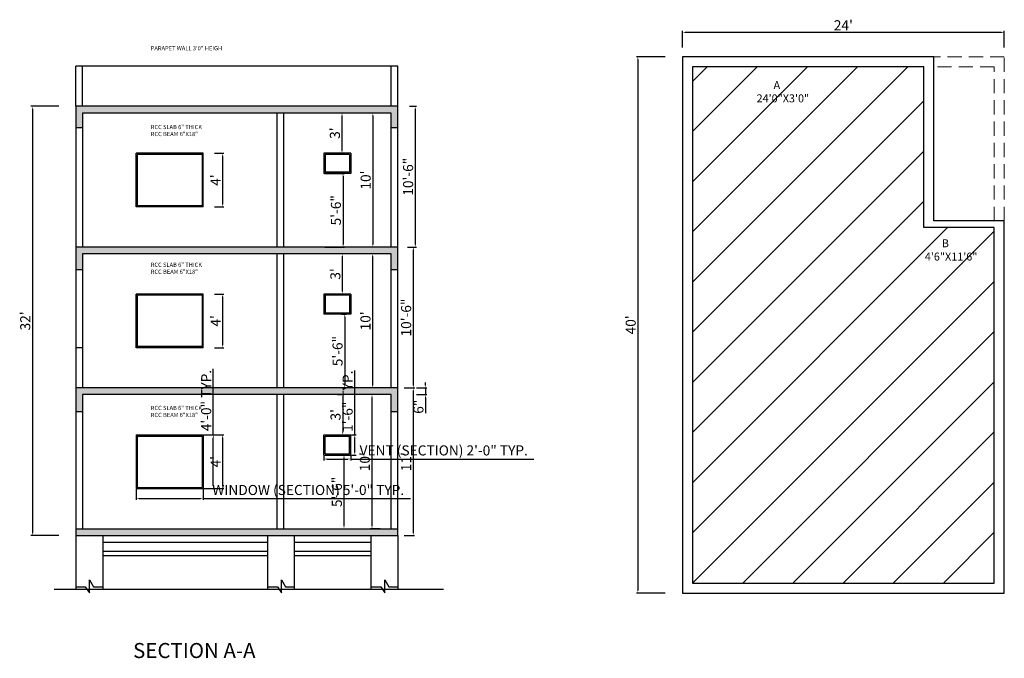
# Model space of a CAD drawing. Units: feet. Extents: x 1398 to 2768, y 682 to 1909.
# Tile 3 of 3: x 1887 to 2768, y 1338 to 1909. Entities that reach past the tile are written whole.
import ezdxf

# ---------------------------------------------------------------- set-up
doc = ezdxf.new("R2010")
doc.units = ezdxf.units.FT
doc.linetypes.add('DASHED', pattern=[19.05, 12.7, -6.35])
for name, color, linetype, lineweight in [('A-ANNO-DIMS', 2, 'Continuous', 18), ('A-ANNO-TEXT', 7, 'Continuous', 18), ('A-AREA', 7, 'Continuous', 25), ('A-AREA-IDEN', 3, 'Continuous', 18), ('A-AREA-OVHD', 8, 'DASHED', 18), ('A-AREA-PATT', 8, 'Continuous', 13), ('A-SECT', 7, 'Continuous', 25), ('A-SECT-PATT', 8, 'Continuous', 13)]:
    doc.layers.add(name, color=color, linetype=linetype, lineweight=lineweight)
doc.styles.get("Standard").update_dxf_attribs({"font": 'arial.ttf'})
doc.dimstyles.new('ISO-25', dxfattribs={"dimtxt": 9, "dimasz": 2.5, "dimexe": 1.25, "dimexo": 0.625, "dimtad": 1, "dimdec": 1, "dimlunit": 3, "dimtxsty": 'Standard', "dimcen": 2.5, "dimadec": 0, "dimazin": 0, "dimtfac": 1, "dimtdec": 1, "dimtmove": 0, "dimatfit": 3, "dimfxl": 1, "dimarcsym": 0})

# ---------------------------------------------------------------- blocks, each defined once
blk = doc.blocks.new('*D5')
at = {"layer": 'A-ANNO-DIMS', "color": 0, "lineweight": -2, "transparency": 16777216}
for p, q in [((1922.38, 1831.85), (1897.57, 1831.85)), ((1898.82, 1829.35), (1898.82, 1450.35)), ((1922.38, 1447.85), (1897.57, 1447.85))]:
    blk.add_line(p, q, dxfattribs=at)
at = {"layer": 'A-ANNO-DIMS', "color": 0, "transparency": 16777216}
for points in [[(1898.4, 1829.35), (1899.24, 1829.35), (1898.82, 1831.85)], [(1898.4, 1450.35), (1899.24, 1450.35), (1898.82, 1447.85)]]:
    blk.add_solid(points, dxfattribs=at)
at = {"layer": 'Defpoints', "color": 0, "transparency": 16777216}
for p in [(1923.01, 1831.85), (1898.82, 1447.85), (1923.01, 1447.85)]:
    blk.add_point(p, dxfattribs=at)
at = {"layer": 'A-ANNO-DIMS', "color": 0, "transparency": 16777216, "insert": (1893.6, 1639.85), "char_height": 9, "attachment_point": 5, "rotation": 90}
blk.add_mtext("32'", dxfattribs=at)
blk = doc.blocks.new('*D6')
at = {"layer": 'A-ANNO-DIMS', "color": 0, "lineweight": -2, "transparency": 16777216}
for p, q in [((2061.73, 1789.85), (2070.25, 1789.85)), ((2069, 1787.35), (2069, 1744.35)), ((2061.73, 1741.85), (2070.25, 1741.85))]:
    blk.add_line(p, q, dxfattribs=at)
at = {"layer": 'A-ANNO-DIMS', "color": 0, "transparency": 16777216}
for points in [[(2068.58, 1787.35), (2069.42, 1787.35), (2069, 1789.85)], [(2068.58, 1744.35), (2069.42, 1744.35), (2069, 1741.85)]]:
    blk.add_solid(points, dxfattribs=at)
at = {"layer": 'Defpoints', "color": 0, "transparency": 16777216}
for p in [(2061.11, 1789.85), (2061.11, 1741.85), (2069, 1741.85)]:
    blk.add_point(p, dxfattribs=at)
at = {"layer": 'A-ANNO-DIMS', "color": 0, "transparency": 16777216, "insert": (2063.88, 1765.85), "char_height": 9, "attachment_point": 5, "rotation": 90}
blk.add_mtext("4'", dxfattribs=at)
blk = doc.blocks.new('*D7')
at = {"layer": 'A-ANNO-DIMS', "color": 0, "lineweight": -2, "transparency": 16777216}
for p, q in [((2061.73, 1663.85), (2070.25, 1663.85)), ((2069, 1661.35), (2069, 1618.35)), ((2061.73, 1615.85), (2070.25, 1615.85))]:
    blk.add_line(p, q, dxfattribs=at)
at = {"layer": 'A-ANNO-DIMS', "color": 0, "transparency": 16777216}
for points in [[(2068.58, 1661.35), (2069.42, 1661.35), (2069, 1663.85)], [(2068.58, 1618.35), (2069.42, 1618.35), (2069, 1615.85)]]:
    blk.add_solid(points, dxfattribs=at)
at = {"layer": 'Defpoints', "color": 0, "transparency": 16777216}
for p in [(2061.11, 1663.85), (2061.11, 1615.85), (2069, 1615.85)]:
    blk.add_point(p, dxfattribs=at)
at = {"layer": 'A-ANNO-DIMS', "color": 0, "transparency": 16777216, "insert": (2063.88, 1639.85), "char_height": 9, "attachment_point": 5, "rotation": 90}
blk.add_mtext("4'", dxfattribs=at)
blk = doc.blocks.new('*D8')
at = {"layer": 'A-ANNO-DIMS', "color": 0, "lineweight": -2, "transparency": 16777216}
for p, q in [((2061.73, 1537.85), (2070.25, 1537.85)), ((2069, 1535.35), (2069, 1492.35)), ((2061.73, 1489.85), (2070.25, 1489.85))]:
    blk.add_line(p, q, dxfattribs=at)
at = {"layer": 'A-ANNO-DIMS', "color": 0, "transparency": 16777216}
for points in [[(2068.58, 1535.35), (2069.42, 1535.35), (2069, 1537.85)], [(2068.58, 1492.35), (2069.42, 1492.35), (2069, 1489.85)]]:
    blk.add_solid(points, dxfattribs=at)
at = {"layer": 'Defpoints', "color": 0, "transparency": 16777216}
for p in [(2061.11, 1537.85), (2061.11, 1489.85), (2069, 1489.85)]:
    blk.add_point(p, dxfattribs=at)
at = {"layer": 'A-ANNO-DIMS', "color": 0, "transparency": 16777216, "insert": (2063.88, 1513.85), "char_height": 9, "attachment_point": 5, "rotation": 90}
blk.add_mtext("4'", dxfattribs=at)
blk = doc.blocks.new('*D9')
at = {"layer": 'A-ANNO-DIMS', "color": 0, "lineweight": -2, "transparency": 16777216}
for p, q in [((2210.76, 1825.85), (2202.2, 1825.85)), ((2203.45, 1823.35), (2203.45, 1708.35)), ((2210.76, 1705.85), (2202.2, 1705.85))]:
    blk.add_line(p, q, dxfattribs=at)
at = {"layer": 'A-ANNO-DIMS', "color": 0, "transparency": 16777216}
for points in [[(2203.04, 1823.35), (2203.87, 1823.35), (2203.45, 1825.85)], [(2203.04, 1708.35), (2203.87, 1708.35), (2203.45, 1705.85)]]:
    blk.add_solid(points, dxfattribs=at)
at = {"layer": 'Defpoints', "color": 0, "transparency": 16777216}
for p in [(2211.39, 1825.85), (2203.45, 1705.85), (2211.39, 1705.85)]:
    blk.add_point(p, dxfattribs=at)
at = {"layer": 'A-ANNO-DIMS', "color": 0, "transparency": 16777216, "insert": (2198.23, 1765.85), "char_height": 9, "attachment_point": 5, "rotation": 90}
blk.add_mtext("10'", dxfattribs=at)
blk = doc.blocks.new('*D10')
at = {"layer": 'A-ANNO-DIMS', "color": 0, "lineweight": -2, "transparency": 16777216}
for p, q in [((2210.57, 1699.85), (2202.01, 1699.85)), ((2203.26, 1697.35), (2203.26, 1582.35)), ((2210.57, 1579.85), (2202.01, 1579.85))]:
    blk.add_line(p, q, dxfattribs=at)
at = {"layer": 'A-ANNO-DIMS', "color": 0, "transparency": 16777216}
for points in [[(2202.84, 1697.35), (2203.68, 1697.35), (2203.26, 1699.85)], [(2202.84, 1582.35), (2203.68, 1582.35), (2203.26, 1579.85)]]:
    blk.add_solid(points, dxfattribs=at)
at = {"layer": 'Defpoints', "color": 0, "transparency": 16777216}
for p in [(2211.2, 1699.85), (2203.26, 1579.85), (2211.2, 1579.85)]:
    blk.add_point(p, dxfattribs=at)
at = {"layer": 'A-ANNO-DIMS', "color": 0, "transparency": 16777216, "insert": (2198.04, 1639.85), "char_height": 9, "attachment_point": 5, "rotation": 90}
blk.add_mtext("10'", dxfattribs=at)
blk = doc.blocks.new('*D11')
at = {"layer": 'A-ANNO-DIMS', "color": 0, "lineweight": -2, "transparency": 16777216}
for p, q in [((2209.99, 1573.85), (2201.43, 1573.85)), ((2202.68, 1571.35), (2202.68, 1456.35)), ((2209.99, 1453.85), (2201.43, 1453.85))]:
    blk.add_line(p, q, dxfattribs=at)
at = {"layer": 'A-ANNO-DIMS', "color": 0, "transparency": 16777216}
for points in [[(2202.27, 1571.35), (2203.1, 1571.35), (2202.68, 1573.85)], [(2202.27, 1456.35), (2203.1, 1456.35), (2202.68, 1453.85)]]:
    blk.add_solid(points, dxfattribs=at)
at = {"layer": 'Defpoints', "color": 0, "transparency": 16777216}
for p in [(2210.62, 1573.85), (2202.68, 1453.85), (2210.62, 1453.85)]:
    blk.add_point(p, dxfattribs=at)
at = {"layer": 'A-ANNO-DIMS', "color": 0, "transparency": 16777216, "insert": (2197.46, 1513.85), "char_height": 9, "attachment_point": 5, "rotation": 90}
blk.add_mtext("10'", dxfattribs=at)
blk = doc.blocks.new('*D12')
at = {"layer": 'A-ANNO-DIMS', "color": 0, "lineweight": -2, "transparency": 16777216}
for p, q in [((2160.35, 1771.85), (2178.06, 1771.85)), ((2176.81, 1769.35), (2176.81, 1708.35)), ((2160.63, 1705.85), (2178.06, 1705.85))]:
    blk.add_line(p, q, dxfattribs=at)
at = {"layer": 'A-ANNO-DIMS', "color": 0, "transparency": 16777216}
for points in [[(2176.39, 1769.35), (2177.23, 1769.35), (2176.81, 1771.85)], [(2176.39, 1708.35), (2177.23, 1708.35), (2176.81, 1705.85)]]:
    blk.add_solid(points, dxfattribs=at)
at = {"layer": 'Defpoints', "color": 0, "transparency": 16777216}
for p in [(2159.72, 1771.85), (2160.01, 1705.85), (2176.81, 1705.85)]:
    blk.add_point(p, dxfattribs=at)
at = {"layer": 'A-ANNO-DIMS', "color": 0, "transparency": 16777216, "insert": (2171.59, 1738.85), "char_height": 9, "attachment_point": 5, "rotation": 90}
blk.add_mtext('5\'-6"', dxfattribs=at)
blk = doc.blocks.new('*D13')
at = {"layer": 'A-ANNO-DIMS', "color": 0, "lineweight": -2, "transparency": 16777216}
for p, q in [((2175.46, 1645.85), (2179.52, 1645.85)), ((2178.27, 1643.35), (2178.27, 1582.35)), ((2175.8, 1579.85), (2179.52, 1579.85))]:
    blk.add_line(p, q, dxfattribs=at)
at = {"layer": 'A-ANNO-DIMS', "color": 0, "transparency": 16777216}
for points in [[(2177.85, 1643.35), (2178.68, 1643.35), (2178.27, 1645.85)], [(2177.85, 1582.35), (2178.68, 1582.35), (2178.27, 1579.85)]]:
    blk.add_solid(points, dxfattribs=at)
at = {"layer": 'Defpoints', "color": 0, "transparency": 16777216}
for p in [(2174.83, 1645.85), (2175.17, 1579.85), (2178.27, 1579.85)]:
    blk.add_point(p, dxfattribs=at)
at = {"layer": 'A-ANNO-DIMS', "color": 0, "transparency": 16777216, "insert": (2173.05, 1612.85), "char_height": 9, "attachment_point": 5, "rotation": 90}
blk.add_mtext('5\'-6"', dxfattribs=at)
blk = doc.blocks.new('*D14')
at = {"layer": 'A-ANNO-DIMS', "color": 0, "lineweight": -2, "transparency": 16777216}
for p, q in [((2177.04, 1519.85), (2178.9, 1519.85)), ((2177.65, 1517.35), (2177.65, 1456.35)), ((2176.52, 1453.85), (2178.9, 1453.85))]:
    blk.add_line(p, q, dxfattribs=at)
at = {"layer": 'A-ANNO-DIMS', "color": 0, "transparency": 16777216}
for points in [[(2177.24, 1517.35), (2178.07, 1517.35), (2177.65, 1519.85)], [(2177.24, 1456.35), (2178.07, 1456.35), (2177.65, 1453.85)]]:
    blk.add_solid(points, dxfattribs=at)
at = {"layer": 'Defpoints', "color": 0, "transparency": 16777216}
for p in [(2176.42, 1519.85), (2175.89, 1453.85), (2177.65, 1453.85)]:
    blk.add_point(p, dxfattribs=at)
at = {"layer": 'A-ANNO-DIMS', "color": 0, "transparency": 16777216, "insert": (2172.43, 1486.85), "char_height": 9, "attachment_point": 5, "rotation": 90}
blk.add_mtext('5\'-6"', dxfattribs=at)
blk = doc.blocks.new('*D15')
at = {"layer": 'A-ANNO-DIMS', "color": 0, "lineweight": -2, "transparency": 16777216}
for p, q in [((2171.88, 1573.85), (2177.74, 1573.85)), ((2176.49, 1571.35), (2176.49, 1540.35)), ((2172.35, 1537.85), (2177.74, 1537.85))]:
    blk.add_line(p, q, dxfattribs=at)
at = {"layer": 'A-ANNO-DIMS', "color": 0, "transparency": 16777216}
for points in [[(2176.07, 1571.35), (2176.91, 1571.35), (2176.49, 1573.85)], [(2176.07, 1540.35), (2176.91, 1540.35), (2176.49, 1537.85)]]:
    blk.add_solid(points, dxfattribs=at)
at = {"layer": 'Defpoints', "color": 0, "transparency": 16777216}
for p in [(2171.25, 1573.85), (2171.72, 1537.85), (2176.49, 1537.85)]:
    blk.add_point(p, dxfattribs=at)
at = {"layer": 'A-ANNO-DIMS', "color": 0, "transparency": 16777216, "insert": (2171.27, 1555.85), "char_height": 9, "attachment_point": 5, "rotation": 90}
blk.add_mtext("3'", dxfattribs=at)
blk = doc.blocks.new('*D16')
at = {"layer": 'A-ANNO-DIMS', "color": 0, "lineweight": -2, "transparency": 16777216}
for p, q in [((2176.37, 1699.85), (2175.07, 1699.85)), ((2176.32, 1666.35), (2176.32, 1697.35)), ((2177.2, 1663.85), (2175.07, 1663.85))]:
    blk.add_line(p, q, dxfattribs=at)
at = {"layer": 'A-ANNO-DIMS', "color": 0, "transparency": 16777216}
for points in [[(2175.9, 1697.35), (2176.74, 1697.35), (2176.32, 1699.85)], [(2175.9, 1666.35), (2176.74, 1666.35), (2176.32, 1663.85)]]:
    blk.add_solid(points, dxfattribs=at)
at = {"layer": 'Defpoints', "color": 0, "transparency": 16777216}
for p in [(2176.32, 1699.85), (2176.99, 1699.85), (2177.82, 1663.85)]:
    blk.add_point(p, dxfattribs=at)
at = {"layer": 'A-ANNO-DIMS', "color": 0, "transparency": 16777216, "insert": (2171.1, 1681.85), "char_height": 9, "attachment_point": 5, "rotation": 90}
blk.add_mtext("3'", dxfattribs=at)
blk = doc.blocks.new('*D17')
at = {"layer": 'A-ANNO-DIMS', "color": 0, "lineweight": -2, "transparency": 16777216}
for p, q in [((2175.42, 1825.85), (2174.67, 1825.85)), ((2175.92, 1792.35), (2175.92, 1823.35)), ((2176.24, 1789.85), (2174.67, 1789.85))]:
    blk.add_line(p, q, dxfattribs=at)
at = {"layer": 'A-ANNO-DIMS', "color": 0, "transparency": 16777216}
for points in [[(2175.51, 1823.35), (2176.34, 1823.35), (2175.92, 1825.85)], [(2175.51, 1792.35), (2176.34, 1792.35), (2175.92, 1789.85)]]:
    blk.add_solid(points, dxfattribs=at)
at = {"layer": 'Defpoints', "color": 0, "transparency": 16777216}
for p in [(2175.92, 1825.85), (2176.04, 1825.85), (2176.87, 1789.85)]:
    blk.add_point(p, dxfattribs=at)
at = {"layer": 'A-ANNO-DIMS', "color": 0, "transparency": 16777216, "insert": (2170.7, 1807.85), "char_height": 9, "attachment_point": 5, "rotation": 90}
blk.add_mtext("3'", dxfattribs=at)
blk = doc.blocks.new('*D18')
at = {"layer": 'A-ANNO-DIMS', "color": 0, "lineweight": -2, "transparency": 16777216}
for p, q in [((2231.49, 1579.85), (2240.83, 1579.85)), ((2239.58, 1577.35), (2239.58, 1450.35)), ((2231.49, 1447.85), (2240.83, 1447.85))]:
    blk.add_line(p, q, dxfattribs=at)
at = {"layer": 'A-ANNO-DIMS', "color": 0, "transparency": 16777216}
for points in [[(2239.17, 1577.35), (2240, 1577.35), (2239.58, 1579.85)], [(2239.17, 1450.35), (2240, 1450.35), (2239.58, 1447.85)]]:
    blk.add_solid(points, dxfattribs=at)
at = {"layer": 'Defpoints', "color": 0, "transparency": 16777216}
for p in [(2230.86, 1579.85), (2230.86, 1447.85), (2239.58, 1447.85)]:
    blk.add_point(p, dxfattribs=at)
at = {"layer": 'A-ANNO-DIMS', "color": 0, "transparency": 16777216, "insert": (2234.44, 1513.85), "char_height": 9, "attachment_point": 5, "rotation": 90}
blk.add_mtext("11'", dxfattribs=at)
blk = doc.blocks.new('*D19')
at = {"layer": 'A-ANNO-DIMS', "color": 0, "lineweight": -2, "transparency": 16777216}
for p, q in [((2234.46, 1705.85), (2240.9, 1705.85)), ((2239.65, 1703.35), (2239.65, 1582.35)), ((2234.46, 1579.85), (2240.9, 1579.85))]:
    blk.add_line(p, q, dxfattribs=at)
at = {"layer": 'A-ANNO-DIMS', "color": 0, "transparency": 16777216}
for points in [[(2239.24, 1703.35), (2240.07, 1703.35), (2239.65, 1705.85)], [(2239.24, 1582.35), (2240.07, 1582.35), (2239.65, 1579.85)]]:
    blk.add_solid(points, dxfattribs=at)
at = {"layer": 'Defpoints', "color": 0, "transparency": 16777216}
for p in [(2233.83, 1705.85), (2233.83, 1579.85), (2239.65, 1579.85)]:
    blk.add_point(p, dxfattribs=at)
at = {"layer": 'A-ANNO-DIMS', "color": 0, "transparency": 16777216, "insert": (2234.43, 1642.85), "char_height": 9, "attachment_point": 5, "rotation": 90}
blk.add_mtext('10\'-6"', dxfattribs=at)
blk = doc.blocks.new('*D20')
at = {"layer": 'A-ANNO-DIMS', "color": 0, "lineweight": -2, "transparency": 16777216}
for p, q in [((2236.21, 1831.85), (2242.66, 1831.85)), ((2241.41, 1829.35), (2241.41, 1708.35)), ((2236.21, 1705.85), (2242.66, 1705.85))]:
    blk.add_line(p, q, dxfattribs=at)
at = {"layer": 'A-ANNO-DIMS', "color": 0, "transparency": 16777216}
for points in [[(2240.99, 1829.35), (2241.82, 1829.35), (2241.41, 1831.85)], [(2240.99, 1708.35), (2241.82, 1708.35), (2241.41, 1705.85)]]:
    blk.add_solid(points, dxfattribs=at)
at = {"layer": 'Defpoints', "color": 0, "transparency": 16777216}
for p in [(2235.58, 1831.85), (2235.58, 1705.85), (2241.41, 1705.85)]:
    blk.add_point(p, dxfattribs=at)
at = {"layer": 'A-ANNO-DIMS', "color": 0, "transparency": 16777216, "insert": (2236.19, 1768.85), "char_height": 9, "attachment_point": 5, "rotation": 90}
blk.add_mtext('10\'-6"', dxfattribs=at)
blk = doc.blocks.new('*D21')
at = {"layer": 'A-ANNO-DIMS', "color": 0, "lineweight": -2, "transparency": 16777216}
for p, q in [((2242.44, 1579.85), (2251.9, 1579.85)), ((2250.65, 1582.35), (2250.65, 1584.85)), ((2250.65, 1579.85), (2250.65, 1573.85)), ((2242.44, 1573.85), (2251.9, 1573.85)), ((2250.65, 1571.35), (2250.65, 1557.2))]:
    blk.add_line(p, q, dxfattribs=at)
at = {"layer": 'A-ANNO-DIMS', "color": 0, "transparency": 16777216}
for points in [[(2250.23, 1582.35), (2251.06, 1582.35), (2250.65, 1579.85)], [(2250.23, 1571.35), (2251.06, 1571.35), (2250.65, 1573.85)]]:
    blk.add_solid(points, dxfattribs=at)
at = {"layer": 'Defpoints', "color": 0, "transparency": 16777216}
for p in [(2241.82, 1579.85), (2241.82, 1573.85), (2250.65, 1573.85)]:
    blk.add_point(p, dxfattribs=at)
at = {"layer": 'A-ANNO-DIMS', "color": 0, "transparency": 16777216, "insert": (2245.43, 1563.03), "char_height": 9, "attachment_point": 5, "rotation": 90}
blk.add_mtext('6"', dxfattribs=at)
blk = doc.blocks.new('*D22')
at = {"layer": 'A-ANNO-DIMS', "color": 0, "lineweight": -2, "transparency": 16777216}
for p, q in [((2480.49, 1884.44), (2480.49, 1899.35)), ((2482.99, 1898.1), (2765.99, 1898.1)), ((2768.49, 1884.44), (2768.49, 1899.35))]:
    blk.add_line(p, q, dxfattribs=at)
at = {"layer": 'A-ANNO-DIMS', "color": 0, "transparency": 16777216}
for points in [[(2482.99, 1898.52), (2482.99, 1897.68), (2480.49, 1898.1)], [(2765.99, 1898.52), (2765.99, 1897.68), (2768.49, 1898.1)]]:
    blk.add_solid(points, dxfattribs=at)
at = {"layer": 'Defpoints', "color": 0, "transparency": 16777216}
for p in [(2768.49, 1898.1), (2480.49, 1883.81), (2768.49, 1883.81)]:
    blk.add_point(p, dxfattribs=at)
at = {"layer": 'A-ANNO-DIMS', "color": 0, "transparency": 16777216, "insert": (2624.49, 1903.24), "char_height": 9, "attachment_point": 5}
blk.add_mtext("24'", dxfattribs=at)
blk = doc.blocks.new('*D23')
at = {"layer": 'A-ANNO-DIMS', "color": 0, "lineweight": -2, "transparency": 16777216}
for p, q in [((2464.94, 1876.29), (2439.34, 1876.29)), ((2440.59, 1873.79), (2440.59, 1398.79)), ((2464.94, 1396.29), (2439.34, 1396.29))]:
    blk.add_line(p, q, dxfattribs=at)
at = {"layer": 'A-ANNO-DIMS', "color": 0, "transparency": 16777216}
for points in [[(2440.17, 1873.79), (2441, 1873.79), (2440.59, 1876.29)], [(2440.17, 1398.79), (2441, 1398.79), (2440.59, 1396.29)]]:
    blk.add_solid(points, dxfattribs=at)
at = {"layer": 'Defpoints', "color": 0, "transparency": 16777216}
for p in [(2465.56, 1876.29), (2440.59, 1396.29), (2465.56, 1396.29)]:
    blk.add_point(p, dxfattribs=at)
at = {"layer": 'A-ANNO-DIMS', "color": 0, "transparency": 16777216, "insert": (2435.37, 1636.29), "char_height": 9, "attachment_point": 5, "rotation": 90}
blk.add_mtext("40'", dxfattribs=at)
blk = doc.blocks.new('SECT-WINDOW-SMALL')
for p, q in [((2159.72, 1537.85), (2183.72, 1537.85)), ((2159.72, 1519.85), (2159.72, 1537.85)), ((2160.72, 1536.85), (2182.72, 1536.85)), ((2160.72, 1520.85), (2160.72, 1536.85)), ((2182.72, 1520.85), (2182.72, 1536.85)), ((2183.72, 1519.85), (2183.72, 1537.85)), ((2159.72, 1519.85), (2183.72, 1519.85)), ((2160.72, 1520.85), (2182.72, 1520.85))]:
    blk.add_line(p, q)
blk = doc.blocks.new('SECT-WINDOW-LARGE')
for p, q in [((0, 48), (60, 48)), ((0, 48), (0, 0)), ((60, 48), (60, 0)), ((0, 0), (60, 0))]:
    blk.add_line(p, q)
blk = doc.blocks.new('*D35')
at = {"layer": 'A-ANNO-DIMS', "color": 0, "lineweight": -2, "transparency": 16777216}
for p, q in [((1991.72, 1489.22), (1991.72, 1479.6)), ((2051.72, 1489.22), (2051.72, 1479.6)), ((1994.22, 1480.85), (2049.22, 1480.85)), ((2051.72, 1480.85), (2237.11, 1480.85))]:
    blk.add_line(p, q, dxfattribs=at)
at = {"layer": 'A-ANNO-DIMS', "color": 0, "transparency": 16777216}
for points in [[(1994.22, 1481.26), (1994.22, 1480.43), (1991.72, 1480.85)], [(2049.22, 1481.26), (2049.22, 1480.43), (2051.72, 1480.85)]]:
    blk.add_solid(points, dxfattribs=at)
at = {"layer": 'Defpoints', "color": 0, "transparency": 16777216}
for p in [(1991.72, 1489.85), (2051.72, 1489.85), (2051.72, 1480.85)]:
    blk.add_point(p, dxfattribs=at)
at = {"layer": 'A-ANNO-DIMS', "color": 0, "transparency": 16777216, "insert": (2145.67, 1487.38), "char_height": 9, "attachment_point": 5}
blk.add_mtext('WINDOW (SECTION) 5\'-0" TYP.', dxfattribs=at)
blk = doc.blocks.new('*D36')
at = {"layer": 'A-ANNO-DIMS', "color": 0, "lineweight": -2, "transparency": 16777216}
for p, q in [((2060.72, 1537.85), (2060.72, 1596.82)), ((2052.35, 1537.85), (2061.97, 1537.85)), ((2060.72, 1492.35), (2060.72, 1535.35)), ((2052.35, 1489.85), (2061.97, 1489.85))]:
    blk.add_line(p, q, dxfattribs=at)
at = {"layer": 'A-ANNO-DIMS', "color": 0, "transparency": 16777216}
for points in [[(2060.3, 1535.35), (2061.14, 1535.35), (2060.72, 1537.85)], [(2060.3, 1492.35), (2061.14, 1492.35), (2060.72, 1489.85)]]:
    blk.add_solid(points, dxfattribs=at)
at = {"layer": 'Defpoints', "color": 0, "transparency": 16777216}
for p in [(2051.72, 1537.85), (2060.72, 1537.85), (2051.72, 1489.85)]:
    blk.add_point(p, dxfattribs=at)
at = {"layer": 'A-ANNO-DIMS', "color": 0, "transparency": 16777216, "insert": (2055.5, 1568.58), "char_height": 9, "attachment_point": 5, "rotation": 90}
blk.add_mtext('4\'-0" TYP.', dxfattribs=at)
blk = doc.blocks.new('*D37')
at = {"layer": 'A-ANNO-DIMS', "color": 0, "lineweight": -2, "transparency": 16777216}
for p, q in [((2159.72, 1519.22), (2159.72, 1515)), ((2162.22, 1516.25), (2181.22, 1516.25)), ((2183.72, 1519.22), (2183.72, 1515)), ((2183.72, 1516.25), (2347.57, 1516.25))]:
    blk.add_line(p, q, dxfattribs=at)
at = {"layer": 'A-ANNO-DIMS', "color": 0, "transparency": 16777216}
for points in [[(2162.22, 1516.66), (2162.22, 1515.83), (2159.72, 1516.25)], [(2181.22, 1516.66), (2181.22, 1515.83), (2183.72, 1516.25)]]:
    blk.add_solid(points, dxfattribs=at)
at = {"layer": 'Defpoints', "color": 0, "transparency": 16777216}
for p in [(2159.72, 1519.85), (2183.72, 1519.85), (2183.72, 1516.25)]:
    blk.add_point(p, dxfattribs=at)
at = {"layer": 'A-ANNO-DIMS', "color": 0, "transparency": 16777216, "insert": (2266.9, 1522.78), "char_height": 9, "attachment_point": 5}
blk.add_mtext('VENT (SECTION) 2\'-0" TYP.', dxfattribs=at)
blk = doc.blocks.new('*D38')
at = {"layer": 'A-ANNO-DIMS', "color": 0, "lineweight": -2, "transparency": 16777216}
for p, q in [((2187.32, 1537.85), (2187.32, 1595.61)), ((2184.35, 1537.85), (2188.57, 1537.85)), ((2187.32, 1522.35), (2187.32, 1535.35)), ((2184.35, 1519.85), (2188.57, 1519.85))]:
    blk.add_line(p, q, dxfattribs=at)
at = {"layer": 'A-ANNO-DIMS', "color": 0, "transparency": 16777216}
for points in [[(2186.9, 1535.35), (2187.74, 1535.35), (2187.32, 1537.85)], [(2186.9, 1522.35), (2187.74, 1522.35), (2187.32, 1519.85)]]:
    blk.add_solid(points, dxfattribs=at)
at = {"layer": 'Defpoints', "color": 0, "transparency": 16777216}
for p in [(2183.72, 1537.85), (2187.32, 1537.85), (2183.72, 1519.85)]:
    blk.add_point(p, dxfattribs=at)
at = {"layer": 'A-ANNO-DIMS', "color": 0, "transparency": 16777216, "insert": (2182.1, 1567.98), "char_height": 9, "attachment_point": 5, "rotation": 90}
blk.add_mtext('1\'-6" TYP.', dxfattribs=at)

msp = doc.modelspace()

# ---------------------------------------------------------------- hatches: boundary and pattern name
at = {"layer": 'A-AREA-PATT'}
h = msp.add_hatch(dxfattribs=at)
h.set_pattern_fill('ANSI31', color=256, scale=10, style=0)
h.set_pattern_definition([(45, (0, -51.56), (-22.45064, 22.45064), [])])
h.paths.add_polyline_path([(2489.49, 1405.29), (2759.49, 1405.29), (2759.49, 1723.29), (2696.49, 1723.29), (2696.49, 1867.29), (2489.49, 1867.29)])
at = {"layer": 'A-SECT-PATT'}
h = msp.add_hatch(color=256, dxfattribs=at)
h.set_gradient(color2=(0, 0, 0), tint=1, name='INVCURVED')
h.paths.add_polyline_path([(1937.72, 1831.85), (1937.72, 1812.9), (1943.72, 1812.9), (1943.72, 1825.85), (2219.72, 1825.85), (2219.72, 1812.9), (2225.72, 1812.9), (2225.72, 1831.85)])
h.paths.add_polyline_path([(2219.72, 1573.85), (2219.72, 1558.91), (2225.72, 1558.91), (2225.72, 1579.85), (1937.72, 1579.85), (1937.72, 1558.91), (1943.72, 1558.91), (1943.72, 1573.85)])
h = msp.add_hatch(color=256, dxfattribs=at)
h.set_gradient(color2=(0, 0, 0), tint=1, name='INVCURVED')
h.paths.add_polyline_path([(1937.72, 1705.85), (1937.72, 1685.82), (1943.72, 1685.82), (1943.72, 1699.85), (2123.72, 1699.85), (2219.72, 1699.85), (2219.72, 1685.82), (2225.72, 1685.82), (2225.72, 1705.85), (2123.72, 1705.85)])
h = msp.add_hatch(color=256, dxfattribs=at)
h.set_gradient(color2=(0, 0, 0), tint=1, name='INVCURVED')
h.paths.add_polyline_path([(2225.72, 1447.85), (2225.72, 1453.85), (2219.72, 1453.85), (1937.72, 1453.85), (1937.72, 1447.85)])

# ---------------------------------------------------------------- linework, layer by layer
at = {"layer": 'A-AREA'}
for p, q in [((2705.49, 1876.29), (2480.49, 1876.29)), ((2480.49, 1876.29), (2480.49, 1396.29)), ((2705.49, 1729.29), (2705.49, 1876.29)), ((2489.49, 1867.29), (2489.49, 1405.29)), ((2696.49, 1867.29), (2489.49, 1867.29)), ((2696.49, 1723.29), (2696.49, 1867.29)), ((2768.49, 1729.29), (2705.49, 1729.29)), ((2768.49, 1396.29), (2768.49, 1729.29)), ((2759.49, 1723.29), (2696.49, 1723.29)), ((2759.49, 1405.29), (2759.49, 1723.29)), ((2489.49, 1405.29), (2759.49, 1405.29)), ((2480.49, 1396.29), (2768.49, 1396.29))]:
    msp.add_line(p, q, dxfattribs=at)
at = {"layer": 'A-AREA-OVHD'}
for p, q in [((2768.49, 1876.29), (2705.49, 1876.29)), ((2768.49, 1729.29), (2768.49, 1876.29)), ((2759.49, 1867.29), (2705.49, 1867.29)), ((2759.49, 1729.29), (2759.49, 1867.29))]:
    msp.add_line(p, q, dxfattribs=at)
at = {"layer": 'A-SECT'}
for p, q in [((2225.72, 1867.85), (1937.72, 1867.85)), ((1937.72, 1831.85), (1937.72, 1867.85)), ((1943.72, 1831.85), (1943.72, 1867.85)), ((2219.72, 1831.85), (2219.72, 1867.85)), ((2225.72, 1831.85), (2225.72, 1867.85)), ((2225.72, 1831.85), (1937.72, 1831.85)), ((1937.72, 1831.85), (1937.72, 1447.85)), ((2219.72, 1825.85), (1943.72, 1825.85)), ((1943.72, 1825.85), (1943.72, 1705.85)), ((2117.72, 1705.85), (2117.72, 1825.85)), ((2123.72, 1705.85), (2123.72, 1825.85)), ((2219.72, 1705.85), (2219.72, 1825.85)), ((2225.72, 1447.85), (2225.72, 1831.85)), ((1937.72, 1812.9), (1943.72, 1812.9)), ((2219.72, 1812.9), (2225.72, 1812.9)), ((1992.72, 1788.85), (1992.72, 1742.85)), ((2050.72, 1788.85), (1992.72, 1788.85)), ((2050.72, 1788.85), (2050.72, 1742.85)), ((2050.72, 1742.85), (1992.72, 1742.85)), ((2123.72, 1705.85), (1937.72, 1705.85)), ((2225.72, 1705.85), (2123.72, 1705.85)), ((1943.72, 1699.85), (1943.72, 1579.85)), ((2123.72, 1699.85), (1943.72, 1699.85)), ((2117.72, 1579.85), (2117.72, 1699.85)), ((2219.72, 1699.85), (2123.72, 1699.85)), ((2123.72, 1579.85), (2123.72, 1699.85)), ((2219.72, 1579.85), (2219.72, 1699.85)), ((1937.72, 1685.82), (1943.72, 1685.82)), ((2219.72, 1685.82), (2225.72, 1685.82)), ((2051.72, 1662.85), (1991.72, 1662.85)), ((1992.72, 1663.85), (1992.72, 1615.85)), ((2050.72, 1663.85), (2050.72, 1615.85)), ((1943.72, 1615.85), (1937.72, 1615.85)), ((2051.72, 1616.85), (1991.72, 1616.85)), ((2225.72, 1579.85), (1937.72, 1579.85)), ((2219.72, 1573.85), (1943.72, 1573.85)), ((1943.72, 1573.85), (1943.72, 1453.85)), ((2117.72, 1453.85), (2117.72, 1573.85)), ((2123.72, 1453.85), (2123.72, 1573.85)), ((2219.72, 1453.85), (2219.72, 1573.85)), ((1937.72, 1558.91), (1943.72, 1558.91)), ((2219.72, 1558.91), (2225.72, 1558.91)), ((1992.72, 1536.85), (1992.72, 1490.85)), ((1992.72, 1536.85), (2050.72, 1536.85)), ((2050.72, 1536.85), (2050.72, 1490.85)), ((1992.72, 1490.85), (2050.72, 1490.85)), ((1937.72, 1453.85), (2219.72, 1453.85)), ((2219.72, 1453.85), (2225.72, 1453.85)), ((2219.72, 1453.85), (2225.72, 1453.85)), ((1937.72, 1447.85), (2225.72, 1447.85)), ((1937.72, 1447.85), (1937.72, 1399.85)), ((1961.72, 1447.85), (1961.72, 1399.85)), ((2109.16, 1447.85), (2109.16, 1399.85)), ((2133.16, 1447.85), (2133.16, 1399.85)), ((2201.72, 1447.85), (2201.72, 1399.85)), ((2225.72, 1447.85), (2225.72, 1399.85)), ((1961.72, 1441.85), (2109.16, 1441.85)), ((2133.16, 1441.85), (2201.72, 1441.85)), ((1961.72, 1433.85), (2109.16, 1433.85)), ((1961.72, 1429.85), (2109.16, 1429.85)), ((2133.16, 1433.85), (2201.72, 1433.85)), ((2133.16, 1429.85), (2201.72, 1429.85)), ((1937.72, 1401.99), (1946.16, 1401.99)), ((1946.16, 1401.99), (1949.8, 1396.37)), ((1949.8, 1396.37), (1949.8, 1408)), ((1949.8, 1408), (1953.44, 1401.99)), ((1953.44, 1401.99), (1961.72, 1401.99)), ((2109.16, 1401.99), (2118.03, 1401.99)), ((2118.03, 1401.99), (2121.67, 1396.37)), ((2121.67, 1396.37), (2121.67, 1408)), ((2121.67, 1408), (2125.31, 1401.99)), ((2125.31, 1401.99), (2133.16, 1401.99)), ((2201.72, 1401.99), (2210.57, 1401.99)), ((2210.57, 1401.99), (2214.22, 1396.37)), ((2214.22, 1396.37), (2214.22, 1408)), ((2214.22, 1408), (2217.85, 1401.99)), ((2217.85, 1401.99), (2225.72, 1401.99)), ((1918.18, 1399.85), (2266.73, 1399.85))]:
    msp.add_line(p, q, dxfattribs=at)

# ---------------------------------------------------------------- block references
at = {"layer": 'A-SECT', "rotation": 180}
for name, p in [('SECT-WINDOW-LARGE', (2051.72, 1789.85)), ('SECT-WINDOW-SMALL', (4343.44, 3309.69)), ('SECT-WINDOW-LARGE', (2051.72, 1663.85)), ('SECT-WINDOW-SMALL', (4343.44, 3183.69))]:
    msp.add_blockref(name, p, dxfattribs=at)
at = {"layer": 'A-SECT'}
for name, p in [('SECT-WINDOW-LARGE', (1991.72, 1489.85)), ('SECT-WINDOW-SMALL', (0, 0))]:
    msp.add_blockref(name, p, dxfattribs=at)

# ---------------------------------------------------------------- texts
at = {"layer": 'A-ANNO-TEXT', "attachment_point": 1}
for s, width, gutter_width, insert, char_height in [('PARAPET WALL 3\'0" HEIGH', 125.5874, 18.82, (2004.77, 1885.75), 3.7635), ('RCC SLAB 6" THICK \\PRCC BEAM 6"X18"', 125.5874, 18.82, (2004.77, 1815.22), 3.7635), ('RCC SLAB 6" THICK \\PRCC BEAM 6"X18"', 125.5874, 18.82, (2004.77, 1691.96), 3.7635), ('RCC SLAB 6" THICK \\PRCC BEAM 6"X18"', 125.5874, 18.82, (2004.77, 1563.84), 3.7635), ('SECTION A-A', 449.1316, 67.3, (1988.93, 1351.62), 13.4591)]:
    msp.add_mtext_dynamic_manual_height_columns(s, width=width, gutter_width=gutter_width, heights=[0], dxfattribs=dict(at, insert=insert, char_height=char_height))
at = {"layer": 'A-AREA-IDEN', "char_height": 7.109, "attachment_point": 1}
for s, insert in [('       A\\P24\'0"X3\'0"', (2546.82, 1854.39)), ('       B\\P4\'6"X11\'6"', (2697.38, 1712.83))]:
    msp.add_mtext_dynamic_manual_height_columns(s, width=237.2218, gutter_width=35.54, heights=[0], dxfattribs=dict(at, insert=insert))

# ---------------------------------------------------------------- dimensions: what is measured, and where the dimension line sits
at = {"layer": 'A-ANNO-DIMS'}
dim = msp.add_linear_dim(base=(2768.49, 1898.1), p1=(2480.49, 1883.81), p2=(2768.49, 1883.81), dimstyle='ISO-25', override={"dimclrd": 0, "dimclre": 0, "dimclrt": 0}, dxfattribs=at)
dim.commit()
dim.dimension.update_dxf_attribs({"geometry": '*D22', "text_midpoint": (2624.49, 1903.24)})
for base, p1, p2, picture, middle in [((2440.59, 1396.29), (2465.56, 1876.29), (2465.56, 1396.29), '*D23', (2435.37, 1636.29)), ((1898.82, 1447.85), (1923.01, 1831.85), (1923.01, 1447.85), '*D5', (1893.6, 1639.85)), ((2175.92, 1825.85), (2176.87, 1789.85), (2176.04, 1825.85), '*D17', (2170.7, 1807.85)), ((2203.45, 1705.85), (2211.39, 1825.85), (2211.39, 1705.85), '*D9', (2198.23, 1765.85)), ((2241.41, 1705.85), (2235.58, 1831.85), (2235.58, 1705.85), '*D20', (2236.19, 1768.85)), ((2069, 1741.85), (2061.11, 1789.85), (2061.11, 1741.85), '*D6', (2063.88, 1765.85)), ((2176.81, 1705.85), (2159.72, 1771.85), (2160.01, 1705.85), '*D12', (2171.59, 1738.85)), ((2239.65, 1579.85), (2233.83, 1705.85), (2233.83, 1579.85), '*D19', (2234.43, 1642.85)), ((2176.32, 1699.85), (2177.82, 1663.85), (2176.99, 1699.85), '*D16', (2171.1, 1681.85)), ((2203.26, 1579.85), (2211.2, 1699.85), (2211.2, 1579.85), '*D10', (2198.04, 1639.85)), ((2069, 1615.85), (2061.11, 1663.85), (2061.11, 1615.85), '*D7', (2063.88, 1639.85)), ((2178.27, 1579.85), (2174.83, 1645.85), (2175.17, 1579.85), '*D13', (2173.05, 1612.85)), ((2239.58, 1447.85), (2230.86, 1579.85), (2230.86, 1447.85), '*D18', (2234.44, 1513.85)), ((2250.65, 1573.85), (2241.82, 1579.85), (2241.82, 1573.85), '*D21', (2245.43, 1563.03)), ((2176.49, 1537.85), (2171.25, 1573.85), (2171.72, 1537.85), '*D15', (2171.27, 1555.85)), ((2202.68, 1453.85), (2210.62, 1573.85), (2210.62, 1453.85), '*D11', (2197.46, 1513.85)), ((2069, 1489.85), (2061.11, 1537.85), (2061.11, 1489.85), '*D8', (2063.88, 1513.85)), ((2177.65, 1453.85), (2176.42, 1519.85), (2175.89, 1453.85), '*D14', (2172.43, 1486.85))]:
    dim = msp.add_linear_dim(base=base, p1=p1, p2=p2, angle=90, dimstyle='ISO-25', override={"dimclrd": 0, "dimclre": 0, "dimclrt": 0}, dxfattribs=at)
    dim.commit()
    dim.dimension.update_dxf_attribs({"geometry": picture, "text_midpoint": middle})
for base, p1, p2, picture, middle in [((2060.72, 1537.85), (2051.72, 1489.85), (2051.72, 1537.85), '*D36', (2055.5, 1568.58)), ((2187.32, 1537.85), (2183.72, 1519.85), (2183.72, 1537.85), '*D38', (2182.1, 1567.98))]:
    dim = msp.add_linear_dim(base=base, p1=p1, p2=p2, angle=90, text='<> TYP.', dimstyle='ISO-25', override={"dimdec": 1, "dimrnd": 0, "dimzin": 1, "dimlunit": 4, "dimfrac": 2}, dxfattribs=at)
    dim.commit()
    dim.dimension.update_dxf_attribs({"geometry": picture, "text_midpoint": middle})
for base, p1, p2, text, picture, middle in [((2183.72, 1516.25), (2159.72, 1519.85), (2183.72, 1519.85), 'VENT (SECTION) <> TYP.', '*D37', (2266.9, 1522.78)), ((2051.72, 1480.85), (1991.72, 1489.85), (2051.72, 1489.85), 'WINDOW (SECTION) <> TYP.', '*D35', (2145.67, 1487.38))]:
    dim = msp.add_linear_dim(base=base, p1=p1, p2=p2, text=text, dimstyle='ISO-25', override={"dimdec": 1, "dimrnd": 0, "dimzin": 1, "dimlunit": 4, "dimfrac": 2}, dxfattribs=at)
    dim.commit()
    dim.dimension.update_dxf_attribs({"geometry": picture, "text_midpoint": middle})

doc.saveas('drawing.dxf')
